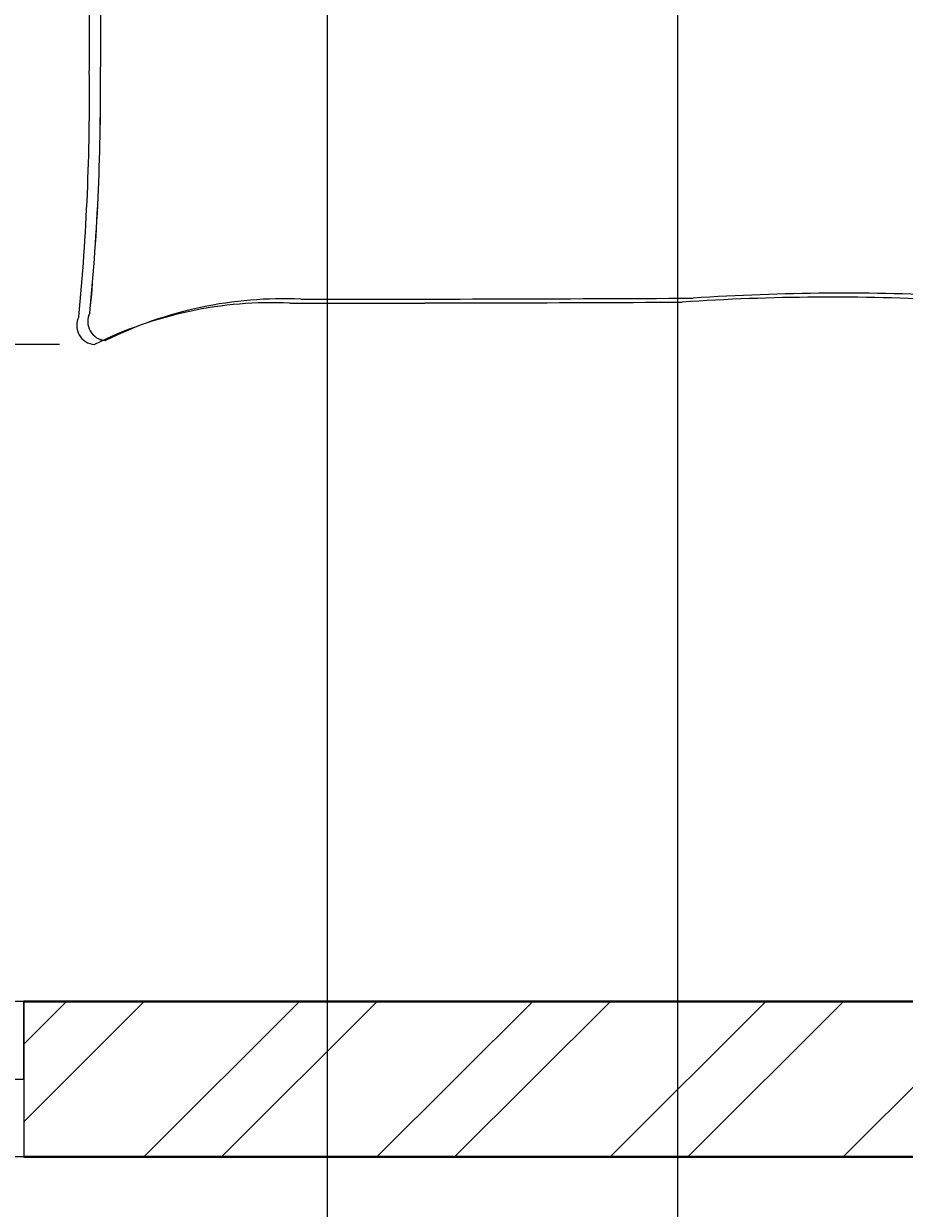
# Model space of a CAD drawing. Units: inches. Extents: x 1601 to 2297, y 1496 to 2631.
# Tile 18 of 57: x 2140 to 2191, y 1632 to 1701. Entities that reach past the tile are written whole.
import ezdxf

# ---------------------------------------------------------------- set-up
doc = ezdxf.new("R2010")
doc.units = ezdxf.units.IN
for name, color, linetype, lineweight in [('A-ANNO-DIMS', 2, 'Continuous', 18), ('A-FURN', 8, 'Continuous', 18), ('A-GLAZ', 161, 'Continuous', 20), ('A-WALL', 7, 'Continuous', 40), ('A-WALL-PATT', 215, 'Continuous', 13)]:
    doc.layers.add(name, color=color, linetype=linetype, lineweight=lineweight)
doc.styles.get("Standard").update_dxf_attribs({"font": 'arial.ttf'})
doc.dimstyles.get("Standard").update_dxf_attribs({"dimtxt": 0.18, "dimasz": 0.18, "dimexe": 0.18, "dimexo": 0.0625, "dimgap": 0.09, "dimtad": 0, "dimtih": 1, "dimtoh": 1, "dimdec": 4, "dimzin": 0, "dimdsep": 46, "dimtxsty": 'Standard', "dimcen": 0.09, "dimadec": 0, "dimazin": 0, "dimtfac": 1, "dimtdec": 4, "dimtofl": 0, "dimtmove": 0, "dimatfit": 3, "dimfxl": 1, "dimtolj": 1, "dimtzin": 0, "dimarcsym": 0})

# ---------------------------------------------------------------- blocks, each defined once
blk = doc.blocks.new('BED-DOUBLE')
for p, q in [((27.746, 52.867), (24.495, 49.162)), ((27.746, 52.867), (24.495, 49.162)), ((27.746, 52.867), (24.495, 49.162)), ((27.746, 52.867), (24.495, 49.162)), ((28.385, 53.096), (25.135, 49.39)), ((28.385, 53.096), (25.135, 49.39)), ((28.385, 53.096), (25.135, 49.39)), ((28.385, 53.096), (25.135, 49.39)), ((29.49, 52.947), (27.746, 52.867, 3.871)), ((29.49, 52.947), (27.746, 52.867, 3.871)), ((29.49, 52.947), (27.746, 52.867, 3.871)), ((29.49, 52.947), (27.746, 52.867, 3.871)), ((28.365, 51.33), (27.746, 52.867)), ((28.365, 51.33), (27.746, 52.867)), ((28.365, 51.33), (27.746, 52.867)), ((28.365, 51.33), (27.746, 52.867)), ((30.13, 53.175), (28.385, 53.096, 3.871)), ((30.13, 53.175), (28.385, 53.096, 3.871)), ((30.13, 53.175), (28.385, 53.096, 3.871)), ((30.13, 53.175), (28.385, 53.096, 3.871)), ((29.004, 51.559), (28.385, 53.096)), ((29.004, 51.558), (28.385, 53.096)), ((29.004, 51.559), (28.385, 53.096)), ((29.004, 51.558), (28.385, 53.096)), ((0, 51.494), (0.639, 51.493)), ((0, 3.475), (0, 51.494)), ((0, 51.494), (0.639, 51.493)), ((0, 3.475), (0, 51.494)), ((0.639, 51.494), (27.249, 51.494)), ((0.639, 51.494), (27.249, 51.494)), ((0.639, 51.493), (27.249, 51.493)), ((0.639, 51.493), (27.249, 51.493)), ((2.173, 3.703), (2.173, 51.494)), ((2.173, 3.703), (2.173, 51.494)), ((2.173, 3.703), (2.173, 51.493)), ((2.173, 3.703), (2.173, 51.493)), ((28.695, 48.461), (29.004, 51.559)), ((28.695, 48.461), (29.004, 51.559)), ((28.695, 48.461), (29.004, 51.558)), ((28.695, 48.461), (29.004, 51.558)), ((0, 51.265), (26.61, 51.265)), ((0, 51.265), (26.61, 51.265)), ((0, 51.265), (26.61, 51.265)), ((0, 51.265), (26.61, 51.265)), ((1.533, 3.475), (1.533, 51.265)), ((1.533, 3.475), (1.533, 51.265)), ((1.533, 3.475), (1.533, 51.265)), ((1.533, 3.475), (1.533, 51.265)), ((16.573, 50.698), (13.434, 49.923)), ((16.573, 50.698), (13.434, 49.922)), ((16.573, 50.698), (13.434, 49.923)), ((16.573, 50.698), (13.434, 49.922)), ((17.212, 50.926), (14.073, 50.151)), ((17.212, 50.926), (14.073, 50.151)), ((17.212, 50.926), (14.073, 50.151)), ((17.212, 50.926), (14.073, 50.151)), ((16.169, 45.566), (16.573, 50.698)), ((16.169, 45.566), (16.573, 50.698)), ((16.169, 45.566), (16.573, 50.698)), ((16.169, 45.566), (16.573, 50.698)), ((16.808, 45.795), (17.212, 50.926)), ((16.808, 45.794), (17.212, 50.926)), ((16.808, 45.795), (17.212, 50.926)), ((16.808, 45.794), (17.212, 50.926)), ((28.055, 48.233), (28.365, 51.33)), ((28.055, 48.233), (28.365, 51.33)), ((28.055, 48.233), (28.365, 51.33)), ((28.055, 48.233), (28.365, 51.33)), ((2.557, 50.112), (2.46, 44.709)), ((2.557, 50.112), (2.46, 44.709)), ((2.557, 50.111), (2.46, 44.709)), ((2.557, 50.111), (2.46, 44.709)), ((2.557, 50.112), (5.768, 49.733)), ((2.557, 50.112), (5.768, 49.733)), ((2.557, 50.111), (5.768, 49.733)), ((2.557, 50.111), (5.768, 49.733)), ((3.196, 50.34), (3.099, 44.938)), ((3.196, 50.34), (3.099, 44.938)), ((3.196, 50.34), (3.099, 44.938)), ((3.196, 50.34), (3.099, 44.938)), ((3.196, 50.34), (6.407, 49.961)), ((3.196, 50.34), (6.407, 49.961)), ((3.196, 50.34), (6.407, 49.961)), ((3.196, 50.34), (6.407, 49.961)), ((5.768, 49.733), (8.338, 50.328)), ((5.768, 49.733), (8.338, 50.328)), ((5.768, 49.733), (8.338, 50.328)), ((5.768, 49.733), (8.338, 50.328)), ((6.407, 49.961), (8.977, 50.557)), ((6.407, 49.961), (8.977, 50.557)), ((6.407, 49.961), (8.977, 50.556)), ((6.407, 49.961), (8.977, 50.556)), ((11.829, 50.112), (8.257, 49.309)), ((11.829, 50.112), (8.257, 49.309)), ((11.829, 50.112), (8.257, 49.309)), ((11.829, 50.112), (8.257, 49.309)), ((8.338, 50.328), (9.384, 49.814)), ((8.338, 50.328), (9.384, 49.814)), ((8.338, 50.328), (9.384, 49.814)), ((8.338, 50.328), (9.384, 49.814)), ((12.468, 50.34), (8.896, 49.538)), ((12.468, 50.34), (8.896, 49.537)), ((12.468, 50.34), (8.896, 49.538)), ((12.468, 50.34), (8.896, 49.537)), ((8.977, 50.557), (10.024, 50.043)), ((8.977, 50.557), (10.024, 50.043)), ((8.977, 50.556), (10.024, 50.042)), ((8.977, 50.556), (10.024, 50.042)), ((13.434, 49.923), (11.829, 50.112)), ((13.434, 49.922), (11.829, 50.112)), ((13.434, 49.923), (11.829, 50.112)), ((13.434, 49.922), (11.829, 50.112)), ((14.073, 50.151), (12.468, 50.34)), ((14.073, 50.151), (12.468, 50.34)), ((14.073, 50.151), (12.468, 50.34)), ((14.073, 50.151), (12.468, 50.34)), ((8.896, 49.538), (6.218, 48.356)), ((8.896, 49.538), (6.218, 48.356)), ((8.896, 49.537), (6.218, 48.356)), ((8.896, 49.537), (6.218, 48.356)), ((25.135, 49.39), (22.968, 46.448)), ((25.135, 49.39), (22.968, 46.448)), ((25.135, 49.39), (22.968, 46.448)), ((25.135, 49.39), (22.968, 46.448)), ((8.257, 49.309), (5.578, 48.128)), ((8.257, 49.309), (5.578, 48.128)), ((8.257, 49.309), (5.578, 48.128)), ((8.257, 49.309), (5.578, 48.128)), ((24.495, 49.162), (22.329, 46.219)), ((24.495, 49.162), (22.329, 46.219)), ((24.495, 49.162), (22.329, 46.219)), ((24.495, 49.162), (22.329, 46.219)), ((28.365, 44.361), (28.055, 48.233)), ((28.365, 44.361), (28.055, 48.233)), ((28.365, 44.361), (28.055, 48.233)), ((28.365, 44.361), (28.055, 48.233)), ((29.004, 44.589), (28.695, 48.461)), ((29.004, 44.589), (28.695, 48.461)), ((29.004, 44.589), (28.695, 48.461)), ((29.004, 44.589), (28.695, 48.461)), ((3.099, 44.938), (3.181, 45.941)), ((3.099, 44.938), (3.181, 45.941)), ((3.099, 44.938), (3.181, 45.94)), ((3.099, 44.938), (3.181, 45.94)), ((3.181, 45.941), (3.709, 42.143)), ((3.181, 45.941), (3.709, 42.143)), ((3.181, 45.94), (3.709, 42.142)), ((3.181, 45.94), (3.709, 42.142)), ((22.329, 46.219), (20.316, 40.644)), ((22.329, 46.219), (20.316, 40.644)), ((22.329, 46.219), (20.317, 40.644)), ((22.329, 46.219), (20.317, 40.644)), ((22.968, 46.448), (20.956, 40.872)), ((22.968, 46.448), (20.956, 40.872)), ((22.968, 46.448), (20.956, 40.872)), ((22.968, 46.448), (20.956, 40.872)), ((2.46, 44.709), (2.542, 45.712)), ((2.46, 44.709), (2.542, 45.712)), ((2.46, 44.709), (2.542, 45.712)), ((2.46, 44.709), (2.542, 45.712)), ((2.542, 45.712), (3.069, 41.914)), ((2.542, 45.712), (3.069, 41.914)), ((2.542, 45.712), (3.069, 41.914)), ((2.542, 45.712), (3.069, 41.914)), ((16.726, 43.606), (16.169, 45.566)), ((16.726, 43.606), (16.169, 45.566)), ((16.726, 43.606), (16.169, 45.566)), ((16.726, 43.606), (16.169, 45.566)), ((17.365, 43.834), (16.808, 45.795)), ((17.365, 43.834), (16.808, 45.795)), ((17.365, 43.834), (16.808, 45.794)), ((17.365, 43.834), (16.808, 45.794)), ((29.468, 41.182), (29.004, 44.589)), ((29.469, 41.182), (29.004, 44.589)), ((29.468, 41.182), (29.004, 44.589)), ((29.469, 41.182), (29.004, 44.589)), ((28.829, 40.954), (28.365, 44.361)), ((28.829, 40.953), (28.365, 44.361)), ((28.829, 40.954), (28.365, 44.361)), ((28.829, 40.953), (28.365, 44.361)), ((16.295, 36.596), (16.726, 43.606)), ((16.295, 36.596), (16.726, 43.606)), ((16.295, 36.596), (16.726, 43.606)), ((16.295, 36.596), (16.726, 43.606)), ((16.934, 36.824), (17.365, 43.834)), ((16.934, 36.824), (17.365, 43.834)), ((16.934, 36.824), (17.365, 43.834)), ((16.934, 36.824), (17.365, 43.834)), ((3.069, 41.914), (4.422, 36.495)), ((3.069, 41.914), (4.422, 36.495)), ((3.069, 41.914), (4.422, 36.495)), ((3.069, 41.914), (4.422, 36.495)), ((3.709, 42.143), (5.061, 36.723)), ((3.709, 42.143), (5.061, 36.723)), ((3.709, 42.142), (5.061, 36.723)), ((3.709, 42.142), (5.061, 36.723)), ((30.397, 39.169), (29.468, 41.182)), ((30.397, 39.169), (29.468, 41.182)), ((30.397, 39.168), (29.469, 41.182)), ((30.397, 39.168), (29.469, 41.182)), ((20.316, 40.644), (17.383, 32.306)), ((20.317, 40.644), (17.383, 32.306)), ((20.316, 40.644), (17.383, 32.306)), ((20.317, 40.644), (17.383, 32.306)), ((20.956, 40.872), (18.022, 32.534)), ((20.956, 40.872), (18.022, 32.534)), ((20.956, 40.872), (18.022, 32.534)), ((20.956, 40.872), (18.022, 32.534)), ((29.758, 38.94), (28.829, 40.954)), ((29.758, 38.94), (28.829, 40.954)), ((29.758, 38.94), (28.829, 40.953)), ((29.758, 38.94), (28.829, 40.953)), ((79.884, 15.292), (79.884, 39.905)), ((79.884, 15.291), (79.884, 39.905)), ((79.884, 15.292), (79.884, 39.905)), ((79.884, 15.291), (79.884, 39.905)), ((3.673, 39.2), (3.078, 37.135)), ((3.673, 39.2), (3.078, 37.135)), ((3.673, 39.2), (3.078, 37.135)), ((3.673, 39.2), (3.078, 37.135)), ((4.313, 39.428), (3.717, 37.363)), ((4.313, 39.428), (3.717, 37.363)), ((4.313, 39.428), (3.718, 37.363)), ((4.313, 39.428), (3.718, 37.363)), ((31.016, 36.691), (30.397, 39.169)), ((31.016, 36.691), (30.397, 39.169)), ((31.016, 36.691), (30.397, 39.168)), ((31.016, 36.691), (30.397, 39.168)), ((79.245, 15.063), (79.245, 39.677)), ((79.245, 15.063), (79.245, 39.677)), ((79.245, 15.063), (79.245, 39.677)), ((79.245, 15.063), (79.245, 39.677)), ((30.377, 36.462), (29.758, 38.94)), ((30.377, 36.462), (29.758, 38.94)), ((30.377, 36.462), (29.758, 38.94)), ((30.377, 36.462), (29.758, 38.94)), ((3.078, 37.135), (2.537, 34.204)), ((3.078, 37.135), (2.537, 34.204)), ((3.078, 37.135), (2.537, 34.204)), ((3.078, 37.135), (2.537, 34.204)), ((3.717, 37.363), (3.176, 34.433)), ((3.718, 37.363), (3.176, 34.433)), ((3.717, 37.363), (3.176, 34.433)), ((3.718, 37.363), (3.176, 34.433)), ((15.628, 32.564), (16.295, 36.596)), ((15.628, 32.564), (16.295, 36.596)), ((15.628, 32.564), (16.295, 36.596)), ((15.628, 32.564), (16.295, 36.596)), ((16.268, 32.792), (16.934, 36.824)), ((16.268, 32.792), (16.934, 36.824)), ((16.268, 32.792), (16.934, 36.824)), ((16.268, 32.792), (16.934, 36.824)), ((24.516, 34.677), (29.004, 36.381)), ((24.516, 34.677), (29.004, 36.381)), ((24.516, 34.677), (29.004, 36.381)), ((24.516, 34.677), (29.004, 36.381)), ((28.365, 36.153), (30.377, 36.462)), ((28.365, 36.152), (30.377, 36.462)), ((28.365, 36.153), (30.377, 36.462)), ((28.365, 36.152), (30.377, 36.462)), ((29.004, 36.381), (31.016, 36.691)), ((29.004, 36.381), (31.016, 36.691)), ((29.004, 36.381), (31.016, 36.691)), ((29.004, 36.381), (31.016, 36.691)), ((23.876, 34.449), (28.365, 36.153)), ((23.876, 34.449), (28.365, 36.153)), ((23.876, 34.449), (28.365, 36.152)), ((23.876, 34.449), (28.365, 36.152)), ((3.176, 34.433), (3.196, 34.112)), ((3.176, 34.433), (3.196, 34.112)), ((3.176, 34.433), (3.196, 34.112)), ((3.176, 34.433), (3.196, 34.112)), ((17.383, 30.259), (23.876, 34.449)), ((17.383, 30.259), (23.876, 34.449)), ((17.383, 30.259), (23.876, 34.449)), ((17.383, 30.259), (23.876, 34.449)), ((18.022, 30.487), (24.516, 34.677)), ((18.022, 30.487), (24.516, 34.677)), ((18.022, 30.487), (24.516, 34.677)), ((18.022, 30.487), (24.516, 34.677)), ((2.537, 34.204), (2.557, 33.883)), ((2.537, 34.204), (2.557, 33.883)), ((2.537, 34.204), (2.557, 33.883)), ((2.537, 34.204), (2.557, 33.883)), ((2.557, 33.883), (2.979, 29.456)), ((2.557, 33.883), (2.979, 29.455)), ((2.557, 33.883), (2.979, 29.456)), ((2.557, 33.883), (2.979, 29.455)), ((3.196, 34.112), (3.618, 29.684)), ((3.196, 34.112), (3.618, 29.684)), ((3.196, 34.112), (3.618, 29.684)), ((3.196, 34.112), (3.618, 29.684)), ((16.739, 30.75), (15.454, 33.821)), ((16.739, 30.75), (15.454, 33.821)), ((16.739, 30.75), (15.454, 33.82)), ((16.739, 30.75), (15.454, 33.82)), ((17.379, 30.978), (16.094, 34.049)), ((17.379, 30.978), (16.094, 34.049)), ((17.379, 30.978), (16.094, 34.049)), ((17.379, 30.978), (16.094, 34.049)), ((17.532, 28.526), (17.379, 30.978)), ((17.532, 28.525), (17.379, 30.978)), ((17.532, 28.526), (17.379, 30.978)), ((17.532, 28.525), (17.379, 30.978)), ((16.893, 28.297), (16.739, 30.75)), ((16.893, 28.297), (16.739, 30.75)), ((16.893, 28.297), (16.739, 30.75)), ((16.893, 28.297), (16.739, 30.75)), ((2.979, 29.456), (2.492, 27.977)), ((2.979, 29.456), (2.492, 27.977)), ((2.979, 29.455), (2.492, 27.976)), ((2.979, 29.455), (2.492, 27.976)), ((3.618, 29.684), (3.131, 28.205)), ((3.618, 29.684), (3.131, 28.205)), ((3.618, 29.684), (3.131, 28.205)), ((3.618, 29.684), (3.131, 28.205)), ((3.131, 28.205), (8.506, 27.962)), ((3.131, 28.205), (8.506, 27.961)), ((3.131, 28.205), (8.506, 27.962)), ((3.131, 28.205), (8.506, 27.961)), ((12.377, 27.436), (14.216, 28.13)), ((12.377, 27.436), (14.217, 28.13)), ((12.377, 27.436), (14.216, 28.13)), ((12.377, 27.436), (14.217, 28.13)), ((13.016, 27.664), (14.856, 28.359)), ((13.016, 27.664), (14.856, 28.359)), ((13.016, 27.664), (14.856, 28.358)), ((13.016, 27.664), (14.856, 28.358)), ((14.216, 28.13), (16.893, 28.297)), ((14.216, 28.13), (16.893, 28.297)), ((14.217, 28.13), (16.893, 28.297)), ((14.217, 28.13), (16.893, 28.297)), ((14.856, 28.359), (17.532, 28.526)), ((14.856, 28.359), (17.532, 28.526)), ((14.856, 28.358), (17.532, 28.525)), ((14.856, 28.358), (17.532, 28.525)), ((2.492, 27.977), (7.867, 27.733)), ((2.492, 27.977), (7.867, 27.733)), ((2.492, 27.976), (7.867, 27.733)), ((2.492, 27.976), (7.867, 27.733)), ((7.867, 27.733), (11.078, 27.355)), ((7.867, 27.733), (11.078, 27.354)), ((7.867, 27.733), (11.078, 27.355)), ((7.867, 27.733), (11.078, 27.354)), ((8.506, 27.962), (11.717, 27.583)), ((8.506, 27.962), (11.717, 27.583)), ((8.506, 27.961), (11.717, 27.583)), ((8.506, 27.961), (11.717, 27.583)), ((11.078, 27.355), (12.377, 27.436)), ((11.078, 27.354), (12.377, 27.436)), ((11.078, 27.355), (12.377, 27.436)), ((11.078, 27.354), (12.377, 27.436)), ((11.717, 27.583), (13.016, 27.664)), ((11.717, 27.583), (13.016, 27.664)), ((11.717, 27.583), (13.016, 27.664)), ((11.717, 27.583), (13.016, 27.664)), ((2.509, 26.211), (7.859, 26.789)), ((2.509, 26.21), (7.859, 26.789)), ((2.509, 26.211), (7.859, 26.789)), ((2.509, 26.21), (7.859, 26.789)), ((7.22, 26.561), (10.401, 27.139)), ((7.22, 26.56), (10.401, 27.139)), ((7.22, 26.561), (10.401, 27.139)), ((7.22, 26.56), (10.401, 27.139)), ((7.859, 26.789), (11.04, 27.367)), ((7.859, 26.789), (11.04, 27.367)), ((7.859, 26.789), (11.04, 27.367)), ((7.859, 26.789), (11.04, 27.367)), ((10.401, 27.139), (11.702, 27.139)), ((10.401, 27.139), (11.702, 27.139)), ((10.401, 27.139), (11.702, 27.139)), ((10.401, 27.139), (11.702, 27.139)), ((11.04, 27.367), (12.341, 27.367)), ((11.04, 27.367), (12.341, 27.367)), ((11.04, 27.367), (12.341, 27.367)), ((11.04, 27.367), (12.341, 27.367)), ((11.702, 27.139), (13.582, 26.561)), ((11.702, 27.139), (13.582, 26.56)), ((11.702, 27.139), (13.582, 26.561)), ((11.702, 27.139), (13.582, 26.56)), ((12.341, 27.367), (14.221, 26.789)), ((12.341, 27.367), (14.221, 26.789)), ((12.341, 27.367), (14.221, 26.789)), ((12.341, 27.367), (14.221, 26.789)), ((14.221, 26.789), (16.902, 26.789)), ((14.221, 26.789), (16.902, 26.789)), ((14.221, 26.789), (16.902, 26.789)), ((14.221, 26.789), (16.902, 26.789)), ((16.902, 26.789), (16.902, 24.332)), ((16.902, 26.789), (16.902, 24.331)), ((16.902, 26.789), (16.902, 24.332)), ((16.902, 26.789), (16.902, 24.331)), ((1.87, 25.982), (7.22, 26.561)), ((1.87, 25.982), (7.22, 26.561)), ((1.87, 25.982), (7.22, 26.56)), ((1.87, 25.982), (7.22, 26.56)), ((3.088, 24.765), (2.509, 26.211)), ((3.088, 24.765), (2.509, 26.211)), ((3.088, 24.765), (2.509, 26.21)), ((3.088, 24.765), (2.509, 26.21)), ((13.582, 26.561), (16.263, 26.561)), ((13.582, 26.561), (16.263, 26.561)), ((13.582, 26.56), (16.263, 26.56)), ((13.582, 26.56), (16.263, 26.56)), ((16.263, 26.561), (16.263, 24.103)), ((16.263, 26.561), (16.263, 24.103)), ((16.263, 26.56), (16.263, 24.103)), ((16.263, 26.56), (16.263, 24.103)), ((2.448, 24.537), (1.87, 25.982)), ((2.448, 24.537), (1.87, 25.982)), ((2.448, 24.537), (1.87, 25.982)), ((2.448, 24.537), (1.87, 25.982)), ((2.943, 20.32), (3.088, 24.765)), ((2.943, 20.319), (3.088, 24.765)), ((2.943, 20.32), (3.088, 24.765)), ((2.943, 20.319), (3.088, 24.765)), ((16.808, 19.612), (17.212, 24.744)), ((16.808, 19.612), (17.212, 24.744)), ((16.808, 19.612), (17.212, 24.744)), ((16.808, 19.612), (17.212, 24.744)), ((2.304, 20.091), (2.448, 24.537)), ((2.304, 20.091), (2.448, 24.537)), ((2.304, 20.091), (2.448, 24.537)), ((2.304, 20.091), (2.448, 24.537)), ((16.263, 24.103), (15.172, 20.959)), ((16.263, 24.103), (15.172, 20.958)), ((16.263, 24.103), (15.172, 20.959)), ((16.263, 24.103), (15.172, 20.958)), ((16.902, 24.332), (15.811, 21.187)), ((16.902, 24.332), (15.811, 21.187)), ((16.902, 24.331), (15.811, 21.187)), ((16.902, 24.331), (15.811, 21.187)), ((16.169, 19.384), (16.573, 24.516)), ((16.169, 19.384), (16.573, 24.516)), ((16.169, 19.383), (16.573, 24.515)), ((16.169, 19.383), (16.573, 24.515)), ((2.304, 19.77), (2.304, 20.091)), ((2.304, 19.769), (2.304, 20.091)), ((2.304, 19.77), (2.304, 20.091)), ((2.304, 19.769), (2.304, 20.091)), ((2.943, 19.998), (2.943, 20.32)), ((2.943, 19.998), (2.943, 20.32)), ((2.943, 19.998), (2.943, 20.319)), ((2.943, 19.998), (2.943, 20.319)), ((3.666, 17.107), (2.943, 19.998)), ((3.666, 17.107), (2.943, 19.998)), ((3.666, 17.107), (2.943, 19.998)), ((3.666, 17.107), (2.943, 19.998)), ((3.027, 16.878), (2.304, 19.77)), ((3.027, 16.878), (2.304, 19.77)), ((3.027, 16.878), (2.304, 19.769)), ((3.027, 16.878), (2.304, 19.769)), ((16.726, 17.423), (16.169, 19.384)), ((16.726, 17.423), (16.169, 19.384)), ((16.726, 17.423), (16.169, 19.383)), ((16.726, 17.423), (16.169, 19.383)), ((17.365, 17.652), (16.808, 19.612)), ((17.365, 17.651), (16.808, 19.612)), ((17.365, 17.652), (16.808, 19.612)), ((17.365, 17.651), (16.808, 19.612)), ((3.955, 12.336), (4.967, 17.83)), ((3.955, 12.336), (4.967, 17.83)), ((3.955, 12.336), (4.967, 17.829)), ((3.955, 12.336), (4.967, 17.829)), ((3.316, 12.108), (4.328, 17.601)), ((3.316, 12.108), (4.328, 17.601)), ((3.316, 12.108), (4.328, 17.601)), ((3.316, 12.108), (4.328, 17.601)), ((16.295, 10.413), (16.726, 17.423)), ((16.295, 10.413), (16.726, 17.423)), ((16.295, 10.413), (16.726, 17.423)), ((16.295, 10.413), (16.726, 17.423)), ((16.934, 10.642), (17.365, 17.652)), ((16.934, 10.642), (17.365, 17.652)), ((16.934, 10.642), (17.365, 17.651)), ((16.934, 10.642), (17.365, 17.651)), ((3.75, 14.855), (3.027, 16.878)), ((3.75, 14.854), (3.027, 16.878)), ((3.75, 14.855), (3.027, 16.878)), ((3.75, 14.854), (3.027, 16.878)), ((4.389, 15.083), (3.666, 17.107)), ((4.389, 15.083), (3.666, 17.107)), ((4.389, 15.083), (3.666, 17.107)), ((4.389, 15.083), (3.666, 17.107)), ((3.666, 8.513), (3.955, 12.336)), ((3.666, 8.513), (3.955, 12.336)), ((3.666, 8.513), (3.955, 12.336)), ((3.666, 8.513), (3.955, 12.336)), ((3.027, 8.285), (3.316, 12.108)), ((3.027, 8.284), (3.316, 12.108)), ((3.027, 8.285), (3.316, 12.108)), ((3.027, 8.284), (3.316, 12.108)), ((15.628, 6.382), (16.295, 10.413)), ((15.628, 6.381), (16.295, 10.413)), ((15.628, 6.382), (16.295, 10.413)), ((15.628, 6.381), (16.295, 10.413)), ((16.268, 6.61), (16.934, 10.642)), ((16.268, 6.61), (16.934, 10.642)), ((16.268, 6.61), (16.934, 10.642)), ((16.268, 6.61), (16.934, 10.642)), ((16.295, 10.413), (16.618, 9.28)), ((16.295, 10.413), (16.618, 9.28)), ((16.295, 10.413), (16.618, 9.28)), ((16.295, 10.413), (16.618, 9.28)), ((16.934, 10.642), (17.257, 9.509)), ((16.934, 10.642), (17.257, 9.508)), ((16.934, 10.642), (17.257, 9.509)), ((16.934, 10.642), (17.257, 9.508)), ((16.618, 9.28), (17.341, 4.184)), ((16.618, 9.28), (17.341, 4.183)), ((16.618, 9.28), (17.341, 4.184)), ((16.618, 9.28), (17.341, 4.183)), ((17.257, 9.509), (17.98, 4.412)), ((17.257, 9.509), (17.98, 4.412)), ((17.257, 9.508), (17.98, 4.412)), ((17.257, 9.508), (17.98, 4.412)), ((3.009, 8.179), (3.027, 8.285)), ((3.009, 8.179), (3.027, 8.285)), ((3.009, 8.179), (3.027, 8.284)), ((3.009, 8.179), (3.027, 8.284)), ((3.648, 8.408), (3.666, 8.513)), ((3.648, 8.407), (3.666, 8.513)), ((3.648, 8.408), (3.666, 8.513)), ((3.648, 8.407), (3.666, 8.513)), ((3.977, 4.127), (3.648, 8.408)), ((3.977, 4.127), (3.648, 8.408)), ((3.977, 4.127), (3.648, 8.407)), ((3.977, 4.127), (3.648, 8.407)), ((3.338, 3.898), (3.009, 8.179)), ((3.338, 3.898), (3.009, 8.179)), ((3.338, 3.898), (3.009, 8.179)), ((3.338, 3.898), (3.009, 8.179)), ((9.594, 5.279), (6.847, 6.291)), ((9.594, 5.279), (6.847, 6.291)), ((9.594, 5.279), (6.847, 6.291)), ((9.594, 5.279), (6.847, 6.291)), ((8.955, 5.051), (6.208, 6.063)), ((8.955, 5.051), (6.208, 6.063)), ((8.955, 5.051), (6.208, 6.063)), ((8.955, 5.051), (6.208, 6.063)), ((12.57, 4.473), (8.955, 5.051)), ((12.57, 4.472), (8.955, 5.051)), ((12.57, 4.473), (8.955, 5.051)), ((12.57, 4.472), (8.955, 5.051)), ((13.209, 4.701), (9.594, 5.279)), ((13.209, 4.701), (9.594, 5.279)), ((13.209, 4.701), (9.594, 5.279)), ((13.209, 4.701), (9.594, 5.279)), ((9.739, 4.267), (10.751, 4.846)), ((9.739, 4.267), (10.751, 4.846)), ((9.739, 4.267), (10.751, 4.845)), ((9.739, 4.267), (10.751, 4.845)), ((14.799, 4.99), (13.209, 4.701)), ((14.799, 4.99), (13.209, 4.701)), ((14.799, 4.99), (13.209, 4.701)), ((14.799, 4.99), (13.209, 4.701)), ((17.98, 4.412), (14.799, 4.99)), ((17.98, 4.412), (14.799, 4.99)), ((17.98, 4.412), (14.799, 4.99)), ((17.98, 4.412), (14.799, 4.99)), ((3.316, 3.894), (6.497, 4.473)), ((3.316, 3.894), (6.497, 4.473)), ((3.316, 3.894), (6.497, 4.472)), ((3.316, 3.894), (6.497, 4.472)), ((3.955, 4.123), (7.136, 4.701)), ((3.955, 4.123), (7.136, 4.701)), ((3.955, 4.123), (7.136, 4.701)), ((3.955, 4.123), (7.136, 4.701)), ((6.497, 4.473), (9.099, 4.039)), ((6.497, 4.473), (9.099, 4.039)), ((6.497, 4.472), (9.099, 4.039)), ((6.497, 4.472), (9.099, 4.039)), ((7.136, 4.701), (9.739, 4.267)), ((7.136, 4.701), (9.739, 4.267)), ((7.136, 4.701), (9.739, 4.267)), ((7.136, 4.701), (9.739, 4.267)), ((9.099, 4.039), (10.112, 4.617)), ((9.099, 4.039), (10.112, 4.617)), ((9.099, 4.039), (10.112, 4.617)), ((9.099, 4.039), (10.112, 4.617)), ((14.16, 4.762), (12.57, 4.473)), ((14.16, 4.762), (12.57, 4.472)), ((14.16, 4.762), (12.57, 4.473)), ((14.16, 4.762), (12.57, 4.472)), ((17.341, 4.184), (14.16, 4.762)), ((17.341, 4.183), (14.16, 4.762)), ((17.341, 4.184), (14.16, 4.762)), ((17.341, 4.183), (14.16, 4.762)), ((18.11, 3.475), (0, 3.475)), ((18.11, 3.475), (0, 3.475)), ((18.11, 3.475), (0, 3.475)), ((18.11, 3.475), (0, 3.475)), ((18.75, 3.703), (0.639, 3.703)), ((18.75, 3.703), (0.639, 3.703)), ((18.75, 3.703), (0.639, 3.703)), ((18.75, 3.703), (0.639, 3.703))]:
    blk.add_line(p, q)
for centre, radius, start, end in [((68.666, 76.157), 23.065, 267.47136, 296.46809), ((68.666, 76.157), 23.065, 267.47136, 296.46809), ((68.666, 76.157), 23.065, 267.47136, 296.46809), ((68.666, 76.157), 23.065, 267.47136, 296.46809), ((69.306, 76.385), 23.065, 267.47136, 296.46809), ((69.306, 76.385), 23.065, 267.47136, 296.46809), ((69.306, 76.385), 23.065, 267.47136, 296.46809), ((69.306, 76.385), 23.065, 267.47136, 296.46809), ((78.87, 54.41), 1.102, 332.65876, 86.02002), ((78.87, 54.409), 1.102, 332.65876, 86.02002), ((78.87, 54.41), 1.102, 332.65876, 86.02002), ((78.87, 54.409), 1.102, 332.65876, 86.02002), ((79.509, 54.638), 1.102, 332.65876, 86.02002), ((79.509, 54.638), 1.102, 332.65876, 86.02002), ((79.509, 54.638), 1.102, 332.65876, 86.02002), ((79.509, 54.638), 1.102, 332.65876, 86.02002), ((212.916, 41.38), 133.04, 174.4998, 180.63509), ((212.916, 41.38), 133.04, 174.4998, 180.63509), ((212.916, 41.38), 133.04, 174.4998, 180.63509), ((212.916, 41.38), 133.04, 174.4998, 180.63509), ((212.276, 41.152), 133.04, 174.4998, 180.63509), ((212.277, 41.151), 133.04, 174.4998, 180.63509), ((212.276, 41.152), 133.04, 174.4998, 180.63509), ((212.277, 41.151), 133.04, 174.4998, 180.63509), ((-6.656, 51.327), 36.183, 349.87628, 2.56571), ((-6.656, 51.327), 36.183, 349.87628, 2.56571), ((-6.656, 51.327), 36.183, 349.87628, 2.56571), ((-6.656, 51.327), 36.183, 349.87628, 2.56571), ((36.315, 182.266), 129.499, 266.97912, 273.83645), ((36.315, 182.265), 129.499, 266.97912, 273.83645), ((36.315, 182.266), 129.499, 266.97912, 273.83645), ((36.315, 182.265), 129.499, 266.97912, 273.83645), ((-6.017, 51.555), 36.183, 349.87628, 2.56571), ((-6.017, 51.555), 36.183, 349.87628, 2.56571), ((-6.017, 51.555), 36.183, 349.87628, 2.56571), ((-6.017, 51.555), 36.183, 349.87628, 2.56571), ((36.954, 182.494), 129.499, 266.97912, 273.83645), ((36.954, 182.494), 129.499, 266.97912, 273.83645), ((36.954, 182.494), 129.499, 266.97912, 273.83645), ((36.954, 182.494), 129.499, 266.97912, 273.83645), ((67.821, -4508.744), 4561.858, 90.002168, 90.286887), ((67.821, -4508.744), 4561.858, 90.002168, 90.286887), ((67.821, -4508.744), 4561.858, 90.002168, 90.286887), ((67.821, -4508.744), 4561.858, 90.002168, 90.286887), ((68.461, -4508.515), 4561.858, 90.002168, 90.286887), ((68.461, -4508.515), 4561.858, 90.002168, 90.286887), ((68.461, -4508.516), 4561.858, 90.002168, 90.286887), ((68.461, -4508.516), 4561.858, 90.002168, 90.286887), ((35.066, 43.743), 6.224, 168.6608, 203.73842), ((35.066, 43.743), 6.224, 168.6608, 203.73842), ((35.066, 43.743), 6.224, 168.6608, 203.73842), ((35.066, 43.743), 6.224, 168.6608, 203.73842), ((35.705, 43.972), 6.224, 168.6608, 203.73842), ((35.705, 43.971), 6.224, 168.6608, 203.73842), ((35.705, 43.972), 6.224, 168.6608, 203.73842), ((35.705, 43.971), 6.224, 168.6608, 203.73842), ((1.482, 31.154), 29.654, 10.66171, 19.88058), ((1.482, 31.154), 29.654, 10.66171, 19.88058), ((1.482, 31.153), 29.654, 10.66171, 19.88058), ((1.482, 31.153), 29.654, 10.66171, 19.88058), ((2.121, 31.382), 29.654, 10.66171, 19.88058), ((2.121, 31.382), 29.654, 10.66171, 19.88058), ((2.121, 31.382), 29.654, 10.66171, 19.88058), ((2.121, 31.382), 29.654, 10.66171, 19.88058), ((156.955, 17.984), 129.02, 171.78449, 186.90062), ((156.955, 17.984), 129.02, 171.78449, 186.90062), ((156.955, 17.984), 129.02, 171.78449, 186.90062), ((156.955, 17.984), 129.02, 171.78449, 186.90062), ((30.439, 36.636), 0.185, 250.24637, 1.13765), ((30.439, 36.636), 0.185, 250.24637, 1.13765), ((30.439, 36.636), 0.185, 250.24637, 1.13765), ((30.439, 36.636), 0.185, 250.24637, 1.13765), ((31.079, 36.864), 0.185, 250.24637, 1.13765), ((31.079, 36.864), 0.185, 250.24637, 1.13765), ((31.079, 36.864), 0.185, 250.24637, 1.13765), ((31.079, 36.864), 0.185, 250.24637, 1.13765), ((156.316, 17.756), 129.02, 171.78449, 186.90062), ((156.316, 17.755), 129.02, 171.78449, 186.90062), ((156.316, 17.756), 129.02, 171.78449, 186.90062), ((156.316, 17.755), 129.02, 171.78449, 186.90062), ((182.052, 21.359), 164.969, 176.08655, 186.78213), ((182.052, 21.359), 164.969, 176.08655, 186.78213), ((182.052, 21.358), 164.969, 176.08655, 186.78213), ((182.052, 21.358), 164.969, 176.08655, 186.78213), ((182.692, 21.587), 164.969, 176.08655, 186.78213), ((182.692, 21.587), 164.969, 176.08655, 186.78213), ((182.692, 21.587), 164.969, 176.08655, 186.78213), ((182.692, 21.587), 164.969, 176.08655, 186.78213), ((-23.712, -17.222), 106.459, 13.38322, 17.70533), ((-23.712, -17.222), 106.459, 13.38322, 17.70533), ((-23.712, -17.222), 106.459, 13.38322, 17.70533), ((-23.712, -17.222), 106.459, 13.38322, 17.70533), ((-23.073, -16.994), 106.459, 13.38322, 17.70533), ((-23.073, -16.994), 106.459, 13.38322, 17.70533), ((-23.073, -16.994), 106.459, 13.38322, 17.70533), ((-23.073, -16.994), 106.459, 13.38322, 17.70533), ((201.476, 21.655), 121.759, 182.99578, 189.40907), ((201.476, 21.655), 121.759, 182.99578, 189.40907), ((201.476, 21.655), 121.759, 182.99578, 189.40907), ((201.476, 21.655), 121.759, 182.99578, 189.40907), ((200.837, 21.427), 121.759, 182.99578, 189.40907), ((200.837, 21.426), 121.759, 182.99578, 189.40907), ((200.837, 21.427), 121.759, 182.99578, 189.40907), ((200.837, 21.426), 121.759, 182.99578, 189.40907), ((31.174, -167.308), 170.11, 88.4762, 91.00819), ((31.174, -167.308), 170.11, 88.4762, 91.00819), ((31.174, -167.308), 170.11, 88.4762, 91.00819), ((31.174, -167.308), 170.11, 88.4762, 91.00819), ((31.813, -167.079), 170.11, 88.4762, 91.00819), ((31.813, -167.08), 170.11, 88.4762, 91.00819), ((31.813, -167.079), 170.11, 88.4762, 91.00819), ((31.813, -167.08), 170.11, 88.4762, 91.00819), ((50.614, 484.822), 482.31, 268.22771, 271.71854), ((50.614, 484.822), 482.31, 268.22771, 271.71854), ((50.614, 484.822), 482.31, 268.22771, 271.71854), ((50.614, 484.822), 482.31, 268.22771, 271.71854), ((51.253, 485.051), 482.31, 268.22771, 271.71854), ((51.253, 485.05), 482.31, 268.22771, 271.71854), ((51.253, 485.051), 482.31, 268.22771, 271.71854), ((51.253, 485.05), 482.31, 268.22771, 271.71854), ((65.154, -26.671), 29.634, 76.06484, 88.91125), ((65.154, -26.672), 29.634, 76.06484, 88.91125), ((65.154, -26.671), 29.634, 76.06484, 88.91125), ((65.154, -26.672), 29.634, 76.06484, 88.91125), ((20.096, 85.162), 83.306, 268.72178, 275.60397), ((20.096, 85.161), 83.306, 268.72178, 275.60397), ((20.096, 85.162), 83.306, 268.72178, 275.60397), ((20.096, 85.161), 83.306, 268.72178, 275.60397), ((20.735, 85.39), 83.306, 268.72178, 275.60397), ((20.735, 85.39), 83.306, 268.72178, 275.60397), ((20.736, 85.39), 83.306, 268.72178, 275.60397), ((20.736, 85.39), 83.306, 268.72178, 275.60397), ((64.515, -26.9), 29.634, 76.06484, 88.91125), ((64.515, -26.9), 29.634, 76.06484, 88.91125), ((64.515, -26.9), 29.634, 76.06484, 88.91125), ((64.515, -26.9), 29.634, 76.06484, 88.91125), ((70.915, -21.431), 23.562, 67.97508, 86.652), ((70.915, -21.432), 23.562, 67.97508, 86.652), ((70.915, -21.431), 23.562, 67.97508, 86.652), ((70.915, -21.432), 23.562, 67.97508, 86.652), ((70.276, -21.66), 23.562, 67.97508, 86.652), ((70.276, -21.66), 23.562, 67.97508, 86.652), ((70.276, -21.66), 23.562, 67.97508, 86.652), ((70.276, -21.66), 23.562, 67.97508, 86.652), ((79.718, 1.087), 1.089, 236.17358, 23.47814), ((79.718, 1.087), 1.089, 236.17358, 23.47814), ((79.718, 1.087), 1.089, 236.17358, 23.47814), ((79.718, 1.087), 1.089, 236.17358, 23.47814), ((80.357, 1.316), 1.089, 236.17358, 23.47814), ((80.357, 1.316), 1.089, 236.17358, 23.47814), ((80.357, 1.315), 1.089, 236.17358, 23.47814), ((80.357, 1.315), 1.089, 236.17358, 23.47814)]:
    blk.add_arc(centre, radius, start, end)
blk = doc.blocks.new('WIN-60IN-JAMB9')
for p, q in [((4.5, 60), (0, 60)), ((0, 60), (9, 60)), ((0, 60), (0, 0)), ((4.5, 0), (4.5, 60)), ((9, 60), (9, 0)), ((0, 0), (9, 0)), ((9, 0), (4.5, 0))]:
    blk.add_line(p, q)
blk = doc.blocks.new('*D13')
at = {"layer": 'A-ANNO-DIMS', "color": 0, "lineweight": -2, "transparency": 16777216}
for p, q in [((2142.316, 1738.128), (2129.966, 1738.128)), ((2130.146, 1737.948), (2130.146, 1710.398)), ((2130.146, 1682.484), (2130.146, 1710.034)), ((2142.316, 1682.304), (2129.966, 1682.304))]:
    blk.add_line(p, q, dxfattribs=at)
at = {"layer": 'A-ANNO-DIMS', "color": 0, "transparency": 16777216}
for points in [[(2130.116, 1737.948), (2130.176, 1737.948), (2130.146, 1738.128)], [(2130.116, 1682.484), (2130.176, 1682.484), (2130.146, 1682.304)]]:
    blk.add_solid(points, dxfattribs=at)
at = {"layer": 'Defpoints', "color": 0, "transparency": 16777216}
for p in [(2142.379, 1738.128), (2130.146, 1682.304), (2142.379, 1682.304)]:
    blk.add_point(p, dxfattribs=at)
at = {"layer": 'A-ANNO-DIMS', "color": 0, "transparency": 16777216, "insert": (2130.146, 1710.216), "char_height": 0.18, "attachment_point": 5}
blk.add_mtext('\\A1;56 TYP.', dxfattribs=at)
blk = doc.blocks.new('*D38')
at = {"layer": 'A-ANNO-DIMS', "color": 0, "lineweight": -2, "transparency": 16777216}
for p, q in [((2178.037, 2085.263), (2178.037, 1513.748)), ((2157.799, 2066.513), (2157.799, 1513.748)), ((2157.979, 1513.928), (2167.523, 1513.928)), ((2177.857, 1513.928), (2168.313, 1513.928))]:
    blk.add_line(p, q, dxfattribs=at)
at = {"layer": 'A-ANNO-DIMS', "color": 0, "transparency": 16777216}
for points in [[(2157.979, 1513.958), (2157.979, 1513.898), (2157.799, 1513.928)], [(2177.857, 1513.958), (2177.857, 1513.898), (2178.037, 1513.928)]]:
    blk.add_solid(points, dxfattribs=at)
at = {"layer": 'Defpoints', "color": 0, "transparency": 16777216}
for p in [(2178.037, 2085.325), (2157.799, 2066.575), (2178.037, 1513.928)]:
    blk.add_point(p, dxfattribs=at)
at = {"layer": 'A-ANNO-DIMS', "color": 0, "transparency": 16777216, "insert": (2167.918, 1513.928), "char_height": 0.18, "attachment_point": 5}
blk.add_mtext('\\A1;20.24', dxfattribs=at)

msp = doc.modelspace()

# ---------------------------------------------------------------- hatches: boundary and pattern name
at = {"layer": 'A-WALL-PATT'}
h = msp.add_hatch(dxfattribs=at)
h.set_pattern_fill('ANSI32', color=256)
h.paths.add_polyline_path([(2230.5373, 1861.8254), (2182.5373, 1861.8254), (2182.5373, 1885.3637), (2178.0373, 1885.3637), (2178.0373, 1861.8254), (2166.0373, 1861.8254), (2134.5373, 1861.8254), (2130.0373, 1861.8254), (2130.0373, 1841.4682), (2126.8833, 1841.4682), (2126.8833, 1836.9682), (2130.0373, 1836.9682), (2130.0373, 1822.7302), (2134.5373, 1822.7302), (2134.5373, 1857.3254), (2166.0373, 1857.3254), (2226.0373, 1857.3254), (2226.0373, 1846.1155), (2230.5373, 1846.1155)])
h.paths.add_polyline_path([(2226.0373, 1797.3254), (2134.5373, 1797.3254), (2134.5373, 1800.6636), (2132.2873, 1800.6636), (2130.0373, 1800.6636), (2130.0373, 1797.3254), (2130.0373, 1792.8254), (2167.7264, 1792.8254), (2226.0373, 1792.8254)])
h.paths.add_polyline_path([(2230.5373, 1822.1155), (2226.0373, 1822.1155), (2226.0373, 1760.8563), (2230.5373, 1760.8563)])
h.paths.add_polyline_path([(2230.5373, 1700.8563), (2226.0373, 1700.8563), (2226.0373, 1644.3254), (2140.2517, 1644.3254), (2140.2517, 1635.3254), (2230.5373, 1635.3254)])
h.paths.add_polyline_path([(2080.2517, 1639.8254), (2080.2517, 1644.3254), (2035.5373, 1644.3254), (2035.5373, 1792.8254), (2094.0373, 1792.8254), (2094.0373, 1797.3254), (2094.0373, 1836.9682), (2097.1057, 1836.9682), (2097.1057, 1839.2182), (2097.1057, 1841.4682), (2094.0373, 1841.4682), (2094.0373, 1862.2276), (2089.5373, 1862.2276), (2089.5373, 1797.3254), (2035.5373, 1797.3254), (2035.5373, 1857.3254), (2035.5373, 1885.0916), (2031.0373, 1885.0916), (2031.0373, 1710.3254), (2012.329, 1710.3254), (2012.329, 1701.3254), (2031.0373, 1701.3254), (2031.0373, 1644.3254), (2031.0373, 1635.3254), (2080.2517, 1635.3254)])
h.paths.add_polyline_path([(1836.0373, 1653.2033), (1842.6171, 1653.2033), (1842.6171, 1657.7033), (1842.6171, 1662.2033), (1831.5373, 1662.2033), (1831.5373, 1764.2033), (1835.3881, 1764.2033), (1835.3881, 1766.4533), (1835.3881, 1768.7033), (1831.5373, 1768.7033), (1827.0373, 1768.7033), (1827.0373, 1662.2033), (1827.0373, 1635.3254), (1836.0373, 1635.3254)])
h.paths.add_polyline_path([(1893.0373, 1701.3254), (1907.193, 1701.3254), (1907.193, 1705.8254), (1907.193, 1710.3254), (1893.0373, 1710.3254), (1893.0373, 1819.8254), (1882.6444, 1819.8254), (1882.6444, 1817.5754), (1882.6444, 1815.3254), (1888.5373, 1815.3254), (1888.5373, 1662.2033), (1884.0373, 1662.2033), (1866.6171, 1662.2033), (1866.6171, 1653.2033), (1882.391, 1653.2033), (1884.0373, 1653.2033), (1884.0373, 1635.3254), (1893.0373, 1635.3254)])
h.paths.add_polyline_path([(1739.3335, 1639.8254), (1739.3335, 1644.3254), (1695.0373, 1644.3254), (1695.0373, 1702.0135), (1690.5373, 1702.0135), (1686.0373, 1702.0135), (1686.0373, 1635.3254), (1739.3335, 1635.3254)])
h.paths.add_polyline_path([(1827.0373, 1644.3254), (1799.3335, 1644.3254), (1799.3335, 1635.3254), (1827.0373, 1635.3254)])
h.paths.add_polyline_path([(1695.0373, 1815.3254), (1849.2759, 1815.3254), (1849.2759, 1819.8254), (1807.5373, 1819.8254), (1807.5373, 1879.8254), (1851.1533, 1879.8254), (1851.1533, 1882.0754), (1851.1533, 1884.3254), (1799.3405, 1884.3254), (1799.3405, 1882.0754), (1799.3405, 1879.8254), (1803.0373, 1879.8254), (1803.0373, 1819.8254), (1695.0373, 1819.8254), (1695.0373, 1835.0458), (1690.5373, 1835.0458), (1686.0373, 1835.0458), (1686.0373, 1766.1753), (1695.0373, 1766.1753)])
h.paths.add_polyline_path([(1775.8157, 1884.3254), (1695.0373, 1884.3254), (1695.0373, 1912.9526), (1690.5373, 1912.9526), (1686.0373, 1912.9526), (1686.0373, 1859.0458), (1695.0373, 1859.0458), (1695.0373, 1879.8254), (1775.8157, 1879.8254)])
h.paths.add_polyline_path([(1893.0373, 2031.3254), (1731.5687, 2031.3254), (1731.5687, 2057.4352), (1722.5687, 2057.4352), (1722.5687, 2031.3254), (1686.0373, 2031.3254), (1686.0373, 1972.9526), (1695.0373, 1972.9526), (1695.0373, 2022.3254), (1888.5373, 2022.3254), (1888.5373, 1884.3254), (1883.4996, 1884.3254), (1883.4996, 1879.8254), (1893.0373, 1879.8254), (1893.0373, 1974.3254), (1976.6199, 1974.3254), (1976.6199, 1978.8254), (1968.0373, 1978.8254), (1968.0373, 1983.3254), (1968.0373, 2008.4756), (1963.5373, 2008.4756), (1959.0373, 2008.4756), (1959.0373, 1983.3254), (1893.0373, 1983.3254)])
h.paths.add_polyline_path([(2230.5373, 2140.4745), (2226.0373, 2140.4745), (2226.0373, 2094.3254), (2040.0373, 2094.3254), (2040.0373, 2085.3254), (2178.0373, 2085.3254), (2178.0373, 2065.6965), (2182.5373, 2065.6965), (2182.5373, 2085.3254), (2226.0373, 2085.3254), (2226.0373, 1986.3254), (2211.2679, 1986.3254), (2211.2679, 1981.8254), (2230.5373, 1981.8254)])
h.paths.add_polyline_path([(2187.6292, 1986.3254), (2182.5373, 1986.3254), (2182.5373, 2029.6965), (2178.0373, 2029.6965), (2178.0373, 1986.3254), (2099.05, 1986.3254), (2099.05, 1981.8254), (2178.0373, 1981.8254), (2178.0373, 1969.3637), (2182.5373, 1969.3637), (2182.5373, 1981.8254), (2187.6292, 1981.8254), (2187.6292, 1984.0754)])
h.paths.add_polyline_path([(1807.1169, 1573.5395), (2055.0405, 1573.5395), (2055.0405, 1610.6322), (1807.1169, 1610.6322)], flags=9)
h.paths.add_polyline_path([(1841.1631, 1712.7967), (1870.3957, 1712.7967), (1870.3957, 1731.454), (1841.1631, 1731.454)], flags=9)
h.paths.add_polyline_path([(2144.3862, 1772.185), (2191.0233, 1772.185), (2191.0233, 1790.8423), (2144.3862, 1790.8423)], flags=9)
h.paths.add_polyline_path([(2143.0128, 1827.3312), (2177.9958, 1827.3312), (2177.9958, 1845.9886), (2143.0128, 1845.9886)], flags=25)
h.paths.add_polyline_path([(2041.2439, 1833.5691), (2070.8516, 1833.5691), (2070.8516, 1852.2264), (2041.2439, 1852.2264)], flags=25)
h.paths.add_polyline_path([(2097.2791, 1947.0598), (2134.2061, 1947.0598), (2134.2061, 1965.7171), (2097.2791, 1965.7171)], flags=9)
h.paths.add_polyline_path([(2214.995, 1904.3124), (2214.995, 1942.2899), (2196.3376, 1942.2899), (2196.3376, 1904.3124)], flags=9)
h.paths.add_polyline_path([(2186.6284, 2043.8031), (2219.7935, 2043.8031), (2219.7935, 2062.4605), (2186.6284, 2062.4605)], flags=25)
h.paths.add_polyline_path([(2064.0877, 2031.616), (2097.4949, 2031.616), (2097.4949, 2050.2734), (2064.0877, 2050.2734)], flags=25)
h.paths.add_polyline_path([(1973.1349, 1986.0688), (2008.4009, 1986.0688), (2008.4009, 2004.7261), (1973.1349, 2004.7261)], flags=9)
h.paths.add_polyline_path([(1976.3676, 2106.9635), (2005.7469, 2106.9635), (2005.7469, 2125.6209), (1976.3676, 2125.6209)], flags=9)
h.paths.add_polyline_path([(1991.7852, 2180.4863), (2027.0513, 2180.4863), (2027.0513, 2199.1437), (1991.7852, 2199.1437)], flags=9)
h.paths.add_polyline_path([(2106.1801, 2187.9359), (2152.2101, 2187.9359), (2152.2101, 2206.5932), (2106.1801, 2206.5932)], flags=9)
h.paths.add_polyline_path([(2148.6686, 2262.2542), (2182.318, 2262.2542), (2182.318, 2280.9115), (2148.6686, 2280.9115)], flags=9)
h.paths.add_polyline_path([(2041.6327, 2252.8147), (2071.2405, 2252.8147), (2071.2405, 2271.4721), (2041.6327, 2271.4721)], flags=9)
h.paths.add_polyline_path([(2063.9734, 2375.4265), (2100.9004, 2375.4265), (2100.9004, 2394.0839), (2063.9734, 2394.0839)], flags=9)
h.paths.add_polyline_path([(2216.4955, 2330.9748), (2216.4955, 2370.2654), (2197.8381, 2370.2654), (2197.8381, 2330.9748)], flags=9)
h.paths.add_polyline_path([(2179.1416, 2485.8687), (2212.3067, 2485.8687), (2212.3067, 2504.5261), (2179.1416, 2504.5261)], flags=9)
h.paths.add_polyline_path([(2078.7442, 2471.1516), (2112.1514, 2471.1516), (2112.1514, 2489.809), (2078.7442, 2489.809)], flags=9)
h.paths.add_polyline_path([(1915.9631, 2329.4668), (1952.8902, 2329.4668), (1952.8902, 2348.1241), (1915.9631, 2348.1241)], flags=9)
h.paths.add_polyline_path([(1904.3189, 2499.6709), (1940.4512, 2499.6709), (1940.4512, 2518.3282), (1904.3189, 2518.3282)], flags=9)
h.paths.add_polyline_path([(1892.3665, 2100.4595), (1925.6374, 2100.4595), (1925.6374, 2119.1169), (1892.3665, 2119.1169)], flags=9)
h.paths.add_polyline_path([(1909.2984, 1805.9631), (1946.2254, 1805.9631), (1946.2254, 1824.6205), (1909.2984, 1824.6205)], flags=9)
h.paths.add_polyline_path([(1934.6056, 1658.616), (1970.738, 1658.616), (1970.738, 1677.2733), (1934.6056, 1677.2733)], flags=9)
h.paths.add_polyline_path([(1711.2052, 1789.8902), (1750.0456, 1789.8902), (1750.0456, 1808.5476), (1711.2052, 1808.5476)], flags=25)
h.paths.add_polyline_path([(1742.7874, 1854.6743), (1771.9449, 1854.6743), (1771.9449, 1873.3317), (1742.7874, 1873.3317)], flags=25)
h.paths.add_polyline_path([(1807.3592, 1997.7912), (1850.1116, 1997.7912), (1850.1116, 2016.4486), (1807.3592, 2016.4486)], flags=25)
h.paths.add_polyline_path([(1717.4579, 2237.7844), (1760.2103, 2237.7844), (1760.2103, 2256.4417), (1717.4579, 2256.4417)], flags=9)
h.paths.add_polyline_path([(1780.9285, 2324.0623), (1810.086, 2324.0623), (1810.086, 2342.7197), (1780.9285, 2342.7197)], flags=9)
h.paths.add_polyline_path([(1837.696, 2449.2024), (1866.9286, 2449.2024), (1866.9286, 2467.8598), (1837.696, 2467.8598)], flags=9)
h.paths.add_polyline_path([(1712.7752, 2484.9404), (1751.6156, 2484.9404), (1751.6156, 2503.5977), (1712.7752, 2503.5977)], flags=9)

# ---------------------------------------------------------------- linework, layer by layer
at = {"layer": 'A-WALL'}
for p, q in [((2140.2517, 1644.3254), (2226.0373, 1644.3254)), ((2140.2517, 1635.3254), (2230.5373, 1635.3254))]:
    msp.add_line(p, q, dxfattribs=at)

# ---------------------------------------------------------------- block references
at = {"layer": 'A-FURN', "rotation": 180}
msp.add_blockref('BED-DOUBLE', (2223.9271, 1738.0414), dxfattribs=at)
at = {"layer": 'A-GLAZ', "rotation": 269.999999999997}
msp.add_blockref('WIN-60IN-JAMB9', (2080.2512, 1644.3257), dxfattribs=at)

# ---------------------------------------------------------------- dimensions: what is measured, and where the dimension line sits
at = {"layer": 'A-ANNO-DIMS'}
dim = msp.add_linear_dim(base=(2178.0373, 1513.9279), p1=(2157.799, 2066.5754), p2=(2178.0373, 2085.3254), dimstyle='Standard', override={"dimdec": 2, "dimlfac": 1, "dimrnd": 0, "dimzin": 0, "dimdsep": 46, "dimlunit": 2}, dxfattribs=at)
dim.commit()
dim.dimension.update_dxf_attribs({"geometry": '*D38', "text_midpoint": (2167.9181, 1513.9279)})
dim = msp.add_linear_dim(base=(2130.1464, 1682.3035), p1=(2142.3787, 1738.1281), p2=(2142.3787, 1682.3035), angle=270, text='<> TYP.', dimstyle='Standard', override={"dimdec": 0, "dimlfac": 1, "dimrnd": 0, "dimzin": 0, "dimdsep": 46, "dimlunit": 2}, dxfattribs=at)
dim.commit()
dim.dimension.update_dxf_attribs({"geometry": '*D13', "text_midpoint": (2130.1464, 1710.2158)})

doc.saveas('drawing.dxf')
